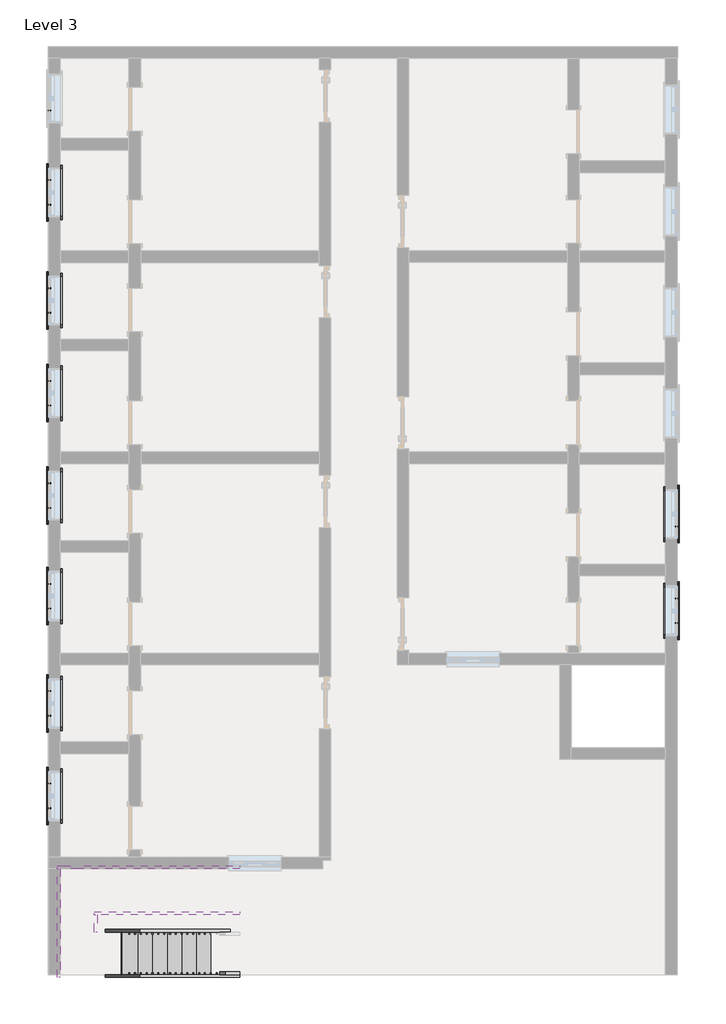
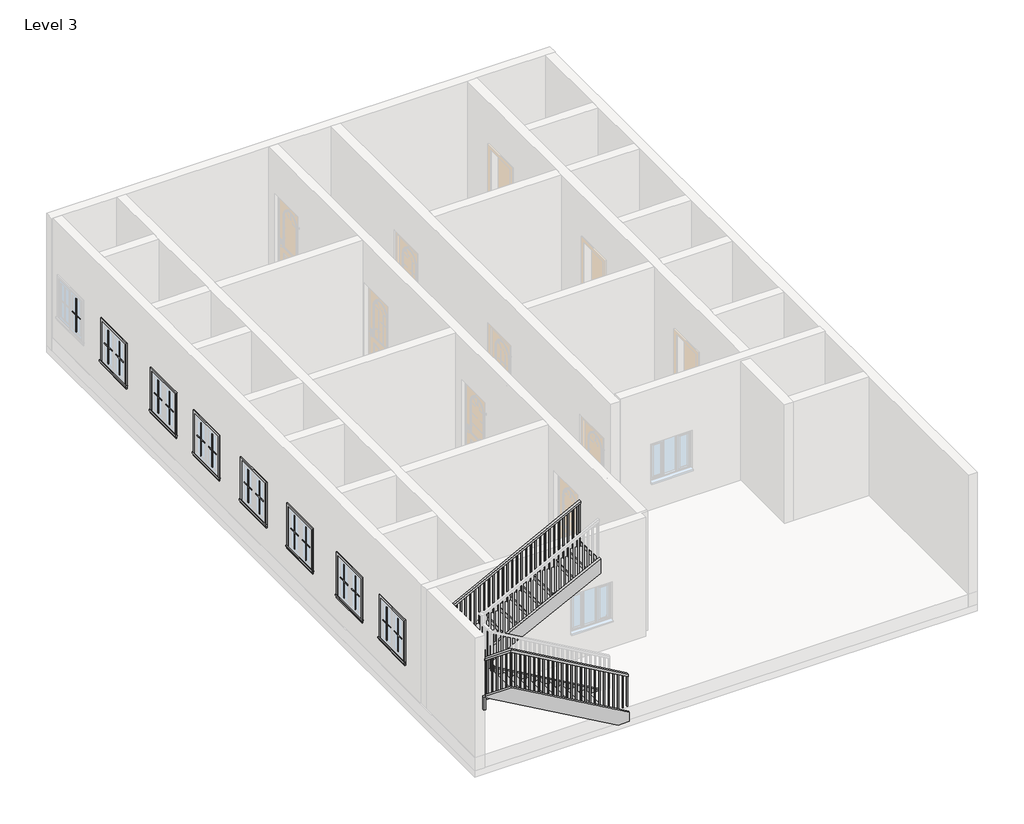
# One storey, part 3 of 4: 36 proxies, 6 members, 1 railing, 1 stair flight.
"""IFC4 building model written with IfcOpenShell, lengths in millimetres."""

from ifc_helpers import new_model, si_unit, frame, origin, place, context, project, spatial, polyline, outline, extrude, faceted_brep, transform, mapped, element, save
from components import muntin_pattern_2x2_muntin_pattern_2x2_b3fe6957, muntin_pattern_2x2_muntin_pattern_2x2_3e0ecaf2, trim_window_exterior_flat_with_sill_41619996, trim_window_interior_flat_picture_frame_51c85655, stair_flight_d547b7c1

model = new_model("IFC4")

# Units and contexts
model_context = context("Model", 3, world=origin())
ifc_project = project(units=[si_unit("LENGTHUNIT", "METRE", prefix="MILLI")], contexts=[model_context])

# Site, building, storey
site = spatial("IfcSite", under=ifc_project)
building = spatial("IfcBuilding", under=site)
storey = spatial("IfcBuildingStorey", under=building, Name="Level 3", Elevation=6096.0)

# Proxies
placement = place(None, origin())
muntin_pattern_2x2_muntin_pattern_2x2_shape = muntin_pattern_2x2_muntin_pattern_2x2_b3fe6957(model_context)
element("IfcBuildingElementProxy", 1, Name="Muntin Pattern_2x2 : Muntin Pattern_2x2", ObjectType="Muntin Pattern_2x2 : Muntin Pattern_2x2", at=placement, inside=storey, context=model_context, shape_type="MappedRepresentation", body=[
    mapped(muntin_pattern_2x2_muntin_pattern_2x2_shape, transform((-6438.8858866, 6882.8274728, 7080.25), x_axis=(0.0, 1.0, 0.0), y_axis=(-1.0, 0.0, 0.0), z_axis=(0.0, 0.0, 1.0))),
])
element("IfcBuildingElementProxy", 2, Name="Muntin Pattern_2x2 : Muntin Pattern_2x2", ObjectType="Muntin Pattern_2x2 : Muntin Pattern_2x2", at=placement, inside=storey, context=model_context, shape_type="MappedRepresentation", body=[
    mapped(muntin_pattern_2x2_muntin_pattern_2x2_shape, transform((-6438.8858866, 5244.5274728, 7080.25), x_axis=(0.0, 1.0, 0.0), y_axis=(-1.0, 0.0, 0.0), z_axis=(0.0, 0.0, 1.0))),
])
element("IfcBuildingElementProxy", 3, Name="Muntin Pattern_2x2 : Muntin Pattern_2x2", ObjectType="Muntin Pattern_2x2 : Muntin Pattern_2x2", at=placement, inside=storey, context=model_context, shape_type="MappedRepresentation", body=[
    mapped(muntin_pattern_2x2_muntin_pattern_2x2_shape, transform((-6438.8858866, 3360.4810874, 7080.25), x_axis=(0.0, 1.0, 0.0), y_axis=(-1.0, 0.0, 0.0), z_axis=(0.0, 0.0, 1.0))),
])
element("IfcBuildingElementProxy", 4, Name="Muntin Pattern_2x2 : Muntin Pattern_2x2", ObjectType="Muntin Pattern_2x2 : Muntin Pattern_2x2", at=placement, inside=storey, context=model_context, shape_type="MappedRepresentation", body=[
    mapped(muntin_pattern_2x2_muntin_pattern_2x2_shape, transform((-6438.8858866, 1745.426343, 7080.25), x_axis=(0.0, 1.0, 0.0), y_axis=(-1.0, 0.0, 0.0), z_axis=(0.0, 0.0, 1.0))),
])
element("IfcBuildingElementProxy", 5, Name="Muntin Pattern_2x2 : Muntin Pattern_2x2", ObjectType="Muntin Pattern_2x2 : Muntin Pattern_2x2", at=placement, inside=storey, context=model_context, shape_type="MappedRepresentation", body=[
    mapped(muntin_pattern_2x2_muntin_pattern_2x2_shape, transform((-6438.8858866, -38.6725272, 7080.25), x_axis=(0.0, 1.0, 0.0), y_axis=(-1.0, 0.0, 0.0), z_axis=(0.0, 0.0, 1.0))),
])
element("IfcBuildingElementProxy", 6, Name="Muntin Pattern_2x2 : Muntin Pattern_2x2", ObjectType="Muntin Pattern_2x2 : Muntin Pattern_2x2", at=placement, inside=storey, context=model_context, shape_type="MappedRepresentation", body=[
    mapped(muntin_pattern_2x2_muntin_pattern_2x2_shape, transform((-6438.8858866, -1791.2725272, 7080.25), x_axis=(0.0, 1.0, 0.0), y_axis=(-1.0, 0.0, 0.0), z_axis=(0.0, 0.0, 1.0))),
])
element("IfcBuildingElementProxy", 7, Name="Muntin Pattern_2x2 : Muntin Pattern_2x2", ObjectType="Muntin Pattern_2x2 : Muntin Pattern_2x2", at=placement, inside=storey, context=model_context, shape_type="MappedRepresentation", body=[
    mapped(muntin_pattern_2x2_muntin_pattern_2x2_shape, transform((-6438.8858866, -3658.1725272, 7080.25), x_axis=(0.0, 1.0, 0.0), y_axis=(-1.0, 0.0, 0.0), z_axis=(0.0, 0.0, 1.0))),
])
element("IfcBuildingElementProxy", 8, Name="Muntin Pattern_2x2 : Muntin Pattern_2x2", ObjectType="Muntin Pattern_2x2 : Muntin Pattern_2x2", at=placement, inside=storey, context=model_context, shape_type="MappedRepresentation", body=[
    mapped(muntin_pattern_2x2_muntin_pattern_2x2_shape, transform((-6438.8858866, -5271.0725272, 7080.25), x_axis=(0.0, 1.0, 0.0), y_axis=(-1.0, 0.0, 0.0), z_axis=(0.0, 0.0, 1.0))),
])
element("IfcBuildingElementProxy", 9, Name="Muntin Pattern_2x2 : Muntin Pattern_2x2", ObjectType="Muntin Pattern_2x2 : Muntin Pattern_2x2", at=placement, inside=storey, context=model_context, shape_type="MappedRepresentation", body=[
    mapped(muntin_pattern_2x2_muntin_pattern_2x2_shape, transform((4489.4641134, -1616.6475272, 7080.25), x_axis=(0.0, -1.0, 0.0), y_axis=(1.0, 0.0, 0.0), z_axis=(0.0, 0.0, 1.0))),
])
muntin_pattern_2x2_muntin_pattern_2x2_2_shape = muntin_pattern_2x2_muntin_pattern_2x2_3e0ecaf2(model_context)
element("IfcBuildingElementProxy", 10, Name="Muntin Pattern_2x2 : Muntin Pattern_2x2", ObjectType="Muntin Pattern_2x2 : Muntin Pattern_2x2", at=placement, inside=storey, context=model_context, shape_type="MappedRepresentation", body=[
    mapped(muntin_pattern_2x2_muntin_pattern_2x2_2_shape, transform((-6438.8858866, 5673.1524728, 7080.25), x_axis=(0.0, -1.0, 0.0), y_axis=(1.0, 0.0, 0.0), z_axis=(0.0, 0.0, 1.0))),
])
element("IfcBuildingElementProxy", 11, Name="Muntin Pattern_2x2 : Muntin Pattern_2x2", ObjectType="Muntin Pattern_2x2 : Muntin Pattern_2x2", at=placement, inside=storey, context=model_context, shape_type="MappedRepresentation", body=[
    mapped(muntin_pattern_2x2_muntin_pattern_2x2_2_shape, transform((-6438.8858866, 3789.1060874, 7080.25), x_axis=(0.0, -1.0, 0.0), y_axis=(1.0, 0.0, 0.0), z_axis=(0.0, 0.0, 1.0))),
])
element("IfcBuildingElementProxy", 12, Name="Muntin Pattern_2x2 : Muntin Pattern_2x2", ObjectType="Muntin Pattern_2x2 : Muntin Pattern_2x2", at=placement, inside=storey, context=model_context, shape_type="MappedRepresentation", body=[
    mapped(muntin_pattern_2x2_muntin_pattern_2x2_2_shape, transform((-6438.8858866, 2174.051343, 7080.25), x_axis=(0.0, -1.0, 0.0), y_axis=(1.0, 0.0, 0.0), z_axis=(0.0, 0.0, 1.0))),
])
element("IfcBuildingElementProxy", 13, Name="Muntin Pattern_2x2 : Muntin Pattern_2x2", ObjectType="Muntin Pattern_2x2 : Muntin Pattern_2x2", at=placement, inside=storey, context=model_context, shape_type="MappedRepresentation", body=[
    mapped(muntin_pattern_2x2_muntin_pattern_2x2_2_shape, transform((-6438.8858866, 389.9524728, 7080.25), x_axis=(0.0, -1.0, 0.0), y_axis=(1.0, 0.0, 0.0), z_axis=(0.0, 0.0, 1.0))),
])
element("IfcBuildingElementProxy", 14, Name="Muntin Pattern_2x2 : Muntin Pattern_2x2", ObjectType="Muntin Pattern_2x2 : Muntin Pattern_2x2", at=placement, inside=storey, context=model_context, shape_type="MappedRepresentation", body=[
    mapped(muntin_pattern_2x2_muntin_pattern_2x2_2_shape, transform((-6438.8858866, -1362.6475272, 7080.25), x_axis=(0.0, -1.0, 0.0), y_axis=(1.0, 0.0, 0.0), z_axis=(0.0, 0.0, 1.0))),
])
element("IfcBuildingElementProxy", 15, Name="Muntin Pattern_2x2 : Muntin Pattern_2x2", ObjectType="Muntin Pattern_2x2 : Muntin Pattern_2x2", at=placement, inside=storey, context=model_context, shape_type="MappedRepresentation", body=[
    mapped(muntin_pattern_2x2_muntin_pattern_2x2_2_shape, transform((-6438.8858866, -3229.5475272, 7080.25), x_axis=(0.0, -1.0, 0.0), y_axis=(1.0, 0.0, 0.0), z_axis=(0.0, 0.0, 1.0))),
])
element("IfcBuildingElementProxy", 16, Name="Muntin Pattern_2x2 : Muntin Pattern_2x2", ObjectType="Muntin Pattern_2x2 : Muntin Pattern_2x2", at=placement, inside=storey, context=model_context, shape_type="MappedRepresentation", body=[
    mapped(muntin_pattern_2x2_muntin_pattern_2x2_2_shape, transform((-6438.8858866, -4842.4475272, 7080.25), x_axis=(0.0, -1.0, 0.0), y_axis=(1.0, 0.0, 0.0), z_axis=(0.0, 0.0, 1.0))),
])
element("IfcBuildingElementProxy", 17, Name="Muntin Pattern_2x2 : Muntin Pattern_2x2", ObjectType="Muntin Pattern_2x2 : Muntin Pattern_2x2", at=placement, inside=storey, context=model_context, shape_type="MappedRepresentation", body=[
    mapped(muntin_pattern_2x2_muntin_pattern_2x2_2_shape, transform((4489.4641134, -2045.2725272, 7080.25), x_axis=(0.0, 1.0, 0.0), y_axis=(-1.0, 0.0, 0.0), z_axis=(0.0, 0.0, 1.0))),
])
element("IfcBuildingElementProxy", 18, Name="Muntin Pattern_2x2 : Muntin Pattern_2x2", ObjectType="Muntin Pattern_2x2 : Muntin Pattern_2x2", at=placement, inside=storey, context=model_context, shape_type="MappedRepresentation", body=[
    mapped(muntin_pattern_2x2_muntin_pattern_2x2_2_shape, transform((4489.4641134, -362.5225272, 7080.25), x_axis=(0.0, 1.0, 0.0), y_axis=(-1.0, 0.0, 0.0), z_axis=(0.0, 0.0, 1.0))),
])
trim_window_exterior_flat_with_sill_shape = trim_window_exterior_flat_with_sill_41619996(model_context)
element("IfcBuildingElementProxy", 19, Name="Trim-Window-Exterior-Flat : with Sill", ObjectType="Trim-Window-Exterior-Flat : with Sill", at=placement, inside=storey, context=model_context, shape_type="MappedRepresentation", body=[
    mapped(trim_window_exterior_flat_with_sill_shape, transform((-6448.4108866, 5458.8399728, 7924.8), x_axis=(0.0, -1.0, 0.0), y_axis=(0.0, 0.0, 1.0), z_axis=(-1.0, 0.0, 0.0))),
])
element("IfcBuildingElementProxy", 20, Name="Trim-Window-Exterior-Flat : with Sill", ObjectType="Trim-Window-Exterior-Flat : with Sill", at=placement, inside=storey, context=model_context, shape_type="MappedRepresentation", body=[
    mapped(trim_window_exterior_flat_with_sill_shape, transform((-6448.4108866, 3574.7935874, 7924.8), x_axis=(0.0, -1.0, 0.0), y_axis=(0.0, 0.0, 1.0), z_axis=(-1.0, 0.0, 0.0))),
])
element("IfcBuildingElementProxy", 21, Name="Trim-Window-Exterior-Flat : with Sill", ObjectType="Trim-Window-Exterior-Flat : with Sill", at=placement, inside=storey, context=model_context, shape_type="MappedRepresentation", body=[
    mapped(trim_window_exterior_flat_with_sill_shape, transform((-6448.4108866, 1959.738843, 7924.8), x_axis=(0.0, -1.0, 0.0), y_axis=(0.0, 0.0, 1.0), z_axis=(-1.0, 0.0, 0.0))),
])
element("IfcBuildingElementProxy", 22, Name="Trim-Window-Exterior-Flat : with Sill", ObjectType="Trim-Window-Exterior-Flat : with Sill", at=placement, inside=storey, context=model_context, shape_type="MappedRepresentation", body=[
    mapped(trim_window_exterior_flat_with_sill_shape, transform((-6448.4108866, 175.6399728, 7924.8), x_axis=(0.0, -1.0, 0.0), y_axis=(0.0, 0.0, 1.0), z_axis=(-1.0, 0.0, 0.0))),
])
element("IfcBuildingElementProxy", 23, Name="Trim-Window-Exterior-Flat : with Sill", ObjectType="Trim-Window-Exterior-Flat : with Sill", at=placement, inside=storey, context=model_context, shape_type="MappedRepresentation", body=[
    mapped(trim_window_exterior_flat_with_sill_shape, transform((-6448.4108866, -1576.9600272, 7924.8), x_axis=(0.0, -1.0, 0.0), y_axis=(0.0, 0.0, 1.0), z_axis=(-1.0, 0.0, 0.0))),
])
element("IfcBuildingElementProxy", 24, Name="Trim-Window-Exterior-Flat : with Sill", ObjectType="Trim-Window-Exterior-Flat : with Sill", at=placement, inside=storey, context=model_context, shape_type="MappedRepresentation", body=[
    mapped(trim_window_exterior_flat_with_sill_shape, transform((-6448.4108866, -3443.8600272, 7924.8), x_axis=(0.0, -1.0, 0.0), y_axis=(0.0, 0.0, 1.0), z_axis=(-1.0, 0.0, 0.0))),
])
element("IfcBuildingElementProxy", 25, Name="Trim-Window-Exterior-Flat : with Sill", ObjectType="Trim-Window-Exterior-Flat : with Sill", at=placement, inside=storey, context=model_context, shape_type="MappedRepresentation", body=[
    mapped(trim_window_exterior_flat_with_sill_shape, transform((-6448.4108866, -5056.7600272, 7924.8), x_axis=(0.0, -1.0, 0.0), y_axis=(0.0, 0.0, 1.0), z_axis=(-1.0, 0.0, 0.0))),
])
element("IfcBuildingElementProxy", 26, Name="Trim-Window-Exterior-Flat : with Sill", ObjectType="Trim-Window-Exterior-Flat : with Sill", at=placement, inside=storey, context=model_context, shape_type="MappedRepresentation", body=[
    mapped(trim_window_exterior_flat_with_sill_shape, transform((4498.9891134, -1830.9600272, 7924.8), x_axis=(0.0, 1.0, 0.0), y_axis=(0.0, 0.0, 1.0), z_axis=(1.0, 0.0, 0.0))),
])
element("IfcBuildingElementProxy", 27, Name="Trim-Window-Exterior-Flat : with Sill", ObjectType="Trim-Window-Exterior-Flat : with Sill", at=placement, inside=storey, context=model_context, shape_type="MappedRepresentation", body=[
    mapped(trim_window_exterior_flat_with_sill_shape, transform((4498.9891134, -148.2100272, 7924.8), x_axis=(0.0, 1.0, 0.0), y_axis=(0.0, 0.0, 1.0), z_axis=(1.0, 0.0, 0.0))),
])
trim_window_interior_flat_picture_frame_shape = trim_window_interior_flat_picture_frame_51c85655(model_context)
element("IfcBuildingElementProxy", 28, Name="Trim-Window-Interior-Flat : Picture Frame", ObjectType="Trim-Window-Interior-Flat : Picture Frame", at=placement, inside=storey, context=model_context, shape_type="MappedRepresentation", body=[
    mapped(trim_window_interior_flat_picture_frame_shape, transform((-6245.2108866, 5458.8399728, 7924.8), x_axis=(0.0, 1.0, 0.0), y_axis=(0.0, 0.0, 1.0), z_axis=(1.0, 0.0, 0.0))),
])
element("IfcBuildingElementProxy", 29, Name="Trim-Window-Interior-Flat : Picture Frame", ObjectType="Trim-Window-Interior-Flat : Picture Frame", at=placement, inside=storey, context=model_context, shape_type="MappedRepresentation", body=[
    mapped(trim_window_interior_flat_picture_frame_shape, transform((-6245.2108866, 3574.7935874, 7924.8), x_axis=(0.0, 1.0, 0.0), y_axis=(0.0, 0.0, 1.0), z_axis=(1.0, 0.0, 0.0))),
])
element("IfcBuildingElementProxy", 30, Name="Trim-Window-Interior-Flat : Picture Frame", ObjectType="Trim-Window-Interior-Flat : Picture Frame", at=placement, inside=storey, context=model_context, shape_type="MappedRepresentation", body=[
    mapped(trim_window_interior_flat_picture_frame_shape, transform((-6245.2108866, 1959.738843, 7924.8), x_axis=(0.0, 1.0, 0.0), y_axis=(0.0, 0.0, 1.0), z_axis=(1.0, 0.0, 0.0))),
])
element("IfcBuildingElementProxy", 31, Name="Trim-Window-Interior-Flat : Picture Frame", ObjectType="Trim-Window-Interior-Flat : Picture Frame", at=placement, inside=storey, context=model_context, shape_type="MappedRepresentation", body=[
    mapped(trim_window_interior_flat_picture_frame_shape, transform((-6245.2108866, 175.6399728, 7924.8), x_axis=(0.0, 1.0, 0.0), y_axis=(0.0, 0.0, 1.0), z_axis=(1.0, 0.0, 0.0))),
])
element("IfcBuildingElementProxy", 32, Name="Trim-Window-Interior-Flat : Picture Frame", ObjectType="Trim-Window-Interior-Flat : Picture Frame", at=placement, inside=storey, context=model_context, shape_type="MappedRepresentation", body=[
    mapped(trim_window_interior_flat_picture_frame_shape, transform((-6245.2108866, -1576.9600272, 7924.8), x_axis=(0.0, 1.0, 0.0), y_axis=(0.0, 0.0, 1.0), z_axis=(1.0, 0.0, 0.0))),
])
element("IfcBuildingElementProxy", 33, Name="Trim-Window-Interior-Flat : Picture Frame", ObjectType="Trim-Window-Interior-Flat : Picture Frame", at=placement, inside=storey, context=model_context, shape_type="MappedRepresentation", body=[
    mapped(trim_window_interior_flat_picture_frame_shape, transform((-6245.2108866, -3443.8600272, 7924.8), x_axis=(0.0, 1.0, 0.0), y_axis=(0.0, 0.0, 1.0), z_axis=(1.0, 0.0, 0.0))),
])
element("IfcBuildingElementProxy", 34, Name="Trim-Window-Interior-Flat : Picture Frame", ObjectType="Trim-Window-Interior-Flat : Picture Frame", at=placement, inside=storey, context=model_context, shape_type="MappedRepresentation", body=[
    mapped(trim_window_interior_flat_picture_frame_shape, transform((-6245.2108866, -5056.7600272, 7924.8), x_axis=(0.0, 1.0, 0.0), y_axis=(0.0, 0.0, 1.0), z_axis=(1.0, 0.0, 0.0))),
])
element("IfcBuildingElementProxy", 35, Name="Trim-Window-Interior-Flat : Picture Frame", ObjectType="Trim-Window-Interior-Flat : Picture Frame", at=placement, inside=storey, context=model_context, shape_type="MappedRepresentation", body=[
    mapped(trim_window_interior_flat_picture_frame_shape, transform((4295.7891134, -1830.9600272, 7924.8), x_axis=(0.0, -1.0, 0.0), y_axis=(0.0, 0.0, 1.0), z_axis=(-1.0, 0.0, 0.0))),
])
element("IfcBuildingElementProxy", 36, Name="Trim-Window-Interior-Flat : Picture Frame", ObjectType="Trim-Window-Interior-Flat : Picture Frame", at=placement, inside=storey, context=model_context, shape_type="MappedRepresentation", body=[
    mapped(trim_window_interior_flat_picture_frame_shape, transform((4295.7891134, -148.2100272, 7924.8), x_axis=(0.0, -1.0, 0.0), y_axis=(0.0, 0.0, 1.0), z_axis=(-1.0, 0.0, 0.0))),
])

# Members
element("IfcMember", 37, ObjectType="Stringer - 2\" Width", at=placement, inside=storey, context=model_context, shape_type="SweptSolid", body=[
    extrude(outline(polyline([(6096.0, -3117.2664982), (6304.974685, -3117.2664982), (7768.7714286, -5678.9107995), (7768.7714286, -6245.2108866), (7741.3177409, -6245.2108866), (6096.0, -3365.9048399), (6096.0, -3117.2664982)])), frame((0.0, -8219.0600272, 0.0), z_axis=(0.0, 1.0, 0.0), x_axis=(0.0, 0.0, 1.0)), (0.0, 0.0, 1.0), 50.8),
])
element("IfcMember", 38, ObjectType="Stringer - 2\" Width", at=placement, inside=storey, context=model_context, shape_type="SweptSolid", body=[
    extrude(outline(polyline([(-6245.2108866, -8219.0600272), (-6296.0108866, -8219.0600272), (-6296.0108866, -6326.7600272), (-6245.2108866, -6326.7600272), (-6245.2108866, -8219.0600272)])), frame((0.0, 0.0, 7463.9714286), z_axis=(0.0, 0.0, 1.0), x_axis=(1.0, 0.0, 0.0)), (0.0, 0.0, 1.0), 304.8),
])
element("IfcMember", 39, ObjectType="Stringer - 2\" Width", at=placement, inside=storey, context=model_context, shape_type="SweptSolid", body=[
    extrude(outline(polyline([(7571.8463219, -6296.0108866), (7463.9714286, -6296.0108866), (7463.9714286, -5835.3420022), (8844.5812084, -3117.2664982), (9186.4466461, -3117.2664982), (7571.8463219, -6296.0108866)])), frame((0.0, -6326.7600272, 0.0), z_axis=(0.0, 1.0, 0.0), x_axis=(0.0, 0.0, 1.0)), (0.0, 0.0, 1.0), 50.8),
])
element("IfcMember", 40, ObjectType="Stringer - 2\" Width", at=placement, inside=storey, context=model_context, shape_type="SweptSolid", body=[
    extrude(outline(polyline([(6096.0, -3117.2664982), (6304.974685, -3117.2664982), (7727.374685, -5606.4664982), (7376.3209476, -5606.4664982), (6096.0, -3365.9048399), (6096.0, -3117.2664982)])), frame((0.0, -7431.6600272, 0.0), z_axis=(0.0, 1.0, 0.0), x_axis=(0.0, 0.0, 1.0)), (0.0, 0.0, 1.0), 50.8),
])
element("IfcMember", 41, ObjectType="Stringer - 2\" Width", at=placement, inside=storey, context=model_context, shape_type="SweptSolid", body=[
    extrude(outline(polyline([(-5606.4664982, -7431.6600272), (-5657.2664982, -7431.6600272), (-5657.2664982, -7126.8600272), (-5606.4664982, -7126.8600272), (-5606.4664982, -7431.6600272)])), frame((0.0, 0.0, 7463.9714286), z_axis=(0.0, 0.0, 1.0), x_axis=(1.0, 0.0, 0.0)), (0.0, 0.0, 1.0), 304.8),
])
element("IfcMember", 42, ObjectType="Stringer - 2\" Width", at=placement, inside=storey, context=model_context, shape_type="SweptSolid", body=[
    extrude(outline(polyline([(7896.287916, -5657.2664982), (7554.4224783, -5657.2664982), (8844.5812084, -3117.2664982), (9186.4466461, -3117.2664982), (7896.287916, -5657.2664982)])), frame((0.0, -7126.8600272, 0.0), z_axis=(0.0, 1.0, 0.0), x_axis=(0.0, 0.0, 1.0)), (0.0, 0.0, 1.0), 50.8),
])

# Railing
element("IfcRailing", 43, ObjectType="Handrail - Rectangular", at=placement, inside=storey, context=model_context, shape_type="SolidModel", body=[
    faceted_brep([(-3117.2664982, -8168.2600272, 7155.5428571), (-3117.2664982, -8168.2600272, 7097.0339009), (-3117.2664982, -8117.4600272, 7097.0339009), (-3117.2664982, -8117.4600272, 7155.5428571), (-5657.2664982, -8168.2600272, 8606.9714286), (-5670.7571716, -8168.2600272, 8556.1714286), (-5670.7571716, -8117.4600272, 8556.1714286), (-5657.2664982, -8117.4600272, 8606.9714286), (-6245.2108866, -8168.2600272, 8606.9714286), (-6245.2108866, -8168.2600272, 8556.1714286), (-6194.4108866, -8117.4600272, 8556.1714286), (-6194.4108866, -8117.4600272, 8606.9714286), (-6245.2108866, -6326.7600272, 8606.9714286), (-6245.2108866, -6326.7600272, 8556.1714286), (-6194.4108866, -6377.5600272, 8556.1714286), (-6194.4108866, -6377.5600272, 8606.9714286), (-5939.4887204, -6326.7600272, 8606.9714286), (-5927.1913462, -6326.7600272, 8556.1714286), (-5927.1913462, -6377.5600272, 8556.1714286), (-5939.4887204, -6377.5600272, 8606.9714286), (-3117.2664982, -6326.7600272, 10058.4), (-3117.2664982, -6377.5600272, 10058.4), (-3117.2664982, -6377.5600272, 10001.2756361), (-3117.2664982, -6326.7600272, 10001.2756361)], [[[0, 1, 2, 3]], [[1, 0, 4, 5]], [[2, 1, 5, 6]], [[3, 2, 6, 7]], [[0, 3, 7, 4]], [[5, 4, 8, 9]], [[6, 5, 9, 10]], [[7, 6, 10, 11]], [[4, 7, 11, 8]], [[9, 8, 12, 13]], [[10, 9, 13, 14]], [[11, 10, 14, 15]], [[8, 11, 15, 12]], [[13, 12, 16, 17]], [[14, 13, 17, 18]], [[15, 14, 18, 19]], [[12, 15, 19, 16]], [[20, 21, 22, 23]], [[17, 16, 20, 23]], [[18, 17, 23, 22]], [[19, 18, 22, 21]], [[16, 19, 21, 20]]]),
    extrude(outline(polyline([(9968.325665, -3181.3358866), (8998.8571429, -3181.3358866), (8998.8571429, -3162.2858866), (9978.1228078, -3162.2858866), (9968.325665, -3181.3358866)])), frame((0.0, -6361.6850272, 0.0), z_axis=(0.0, 1.0, 0.0), x_axis=(0.0, 0.0, 1.0)), (0.0, 0.0, 1.0), 19.05),
    extrude(outline(polyline([(9916.0742364, -3282.9358866), (8998.8571429, -3282.9358866), (8998.8571429, -3263.8858866), (9925.8713793, -3263.8858866), (9916.0742364, -3282.9358866)])), frame((0.0, -6361.6850272, 0.0), z_axis=(0.0, 1.0, 0.0), x_axis=(0.0, 0.0, 1.0)), (0.0, 0.0, 1.0), 19.05),
    extrude(outline(polyline([(9863.8228078, -3384.5358866), (8853.7142857, -3384.5358866), (8853.7142857, -3365.4858866), (9873.6199507, -3365.4858866), (9863.8228078, -3384.5358866)])), frame((0.0, -6361.6850272, 0.0), z_axis=(0.0, 1.0, 0.0), x_axis=(0.0, 0.0, 1.0)), (0.0, 0.0, 1.0), 19.05),
    extrude(outline(polyline([(9811.5713793, -3486.1358866), (8853.7142857, -3486.1358866), (8853.7142857, -3467.0858866), (9821.3685221, -3467.0858866), (9811.5713793, -3486.1358866)])), frame((0.0, -6361.6850272, 0.0), z_axis=(0.0, 1.0, 0.0), x_axis=(0.0, 0.0, 1.0)), (0.0, 0.0, 1.0), 19.05),
    extrude(outline(polyline([(9759.3199507, -3587.7358866), (8853.7142857, -3587.7358866), (8853.7142857, -3568.6858866), (9769.1170935, -3568.6858866), (9759.3199507, -3587.7358866)])), frame((0.0, -6361.6850272, 0.0), z_axis=(0.0, 1.0, 0.0), x_axis=(0.0, 0.0, 1.0)), (0.0, 0.0, 1.0), 19.05),
    extrude(outline(polyline([(9707.0685221, -3689.3358866), (8708.5714286, -3689.3358866), (8708.5714286, -3670.2858866), (9716.865665, -3670.2858866), (9707.0685221, -3689.3358866)])), frame((0.0, -6361.6850272, 0.0), z_axis=(0.0, 1.0, 0.0), x_axis=(0.0, 0.0, 1.0)), (0.0, 0.0, 1.0), 19.05),
    extrude(outline(polyline([(9654.8170935, -3790.9358866), (8708.5714286, -3790.9358866), (8708.5714286, -3771.8858866), (9664.6142364, -3771.8858866), (9654.8170935, -3790.9358866)])), frame((0.0, -6361.6850272, 0.0), z_axis=(0.0, 1.0, 0.0), x_axis=(0.0, 0.0, 1.0)), (0.0, 0.0, 1.0), 19.05),
    extrude(outline(polyline([(9602.565665, -3892.5358866), (8708.5714286, -3892.5358866), (8708.5714286, -3873.4858866), (9612.3628078, -3873.4858866), (9602.565665, -3892.5358866)])), frame((0.0, -6361.6850272, 0.0), z_axis=(0.0, 1.0, 0.0), x_axis=(0.0, 0.0, 1.0)), (0.0, 0.0, 1.0), 19.05),
    extrude(outline(polyline([(9550.3142364, -3994.1358866), (8708.5714286, -3994.1358866), (8708.5714286, -3975.0858866), (9560.1113793, -3975.0858866), (9550.3142364, -3994.1358866)])), frame((0.0, -6361.6850272, 0.0), z_axis=(0.0, 1.0, 0.0), x_axis=(0.0, 0.0, 1.0)), (0.0, 0.0, 1.0), 19.05),
    extrude(outline(polyline([(9498.0628078, -4095.7358866), (8708.5714286, -4095.7358866), (8708.5714286, -4076.6858866), (9507.8599507, -4076.6858866), (9498.0628078, -4095.7358866)])), frame((0.0, -6361.6850272, 0.0), z_axis=(0.0, 1.0, 0.0), x_axis=(0.0, 0.0, 1.0)), (0.0, 0.0, 1.0), 19.05),
    extrude(outline(polyline([(9445.8113793, -4197.3358866), (8563.4285714, -4197.3358866), (8563.4285714, -4178.2858866), (9455.6085221, -4178.2858866), (9445.8113793, -4197.3358866)])), frame((0.0, -6361.6850272, 0.0), z_axis=(0.0, 1.0, 0.0), x_axis=(0.0, 0.0, 1.0)), (0.0, 0.0, 1.0), 19.05),
    extrude(outline(polyline([(9393.5599507, -4298.9358866), (8563.4285714, -4298.9358866), (8563.4285714, -4279.8858866), (9403.3570935, -4279.8858866), (9393.5599507, -4298.9358866)])), frame((0.0, -6361.6850272, 0.0), z_axis=(0.0, 1.0, 0.0), x_axis=(0.0, 0.0, 1.0)), (0.0, 0.0, 1.0), 19.05),
    extrude(outline(polyline([(9341.3085221, -4400.5358866), (8418.2857143, -4400.5358866), (8418.2857143, -4381.4858866), (9351.105665, -4381.4858866), (9341.3085221, -4400.5358866)])), frame((0.0, -6361.6850272, 0.0), z_axis=(0.0, 1.0, 0.0), x_axis=(0.0, 0.0, 1.0)), (0.0, 0.0, 1.0), 19.05),
    extrude(outline(polyline([(9289.0570935, -4502.1358866), (8418.2857143, -4502.1358866), (8418.2857143, -4483.0858866), (9298.8542364, -4483.0858866), (9289.0570935, -4502.1358866)])), frame((0.0, -6361.6850272, 0.0), z_axis=(0.0, 1.0, 0.0), x_axis=(0.0, 0.0, 1.0)), (0.0, 0.0, 1.0), 19.05),
    extrude(outline(polyline([(9236.805665, -4603.7358866), (8418.2857143, -4603.7358866), (8418.2857143, -4584.6858866), (9246.6028078, -4584.6858866), (9236.805665, -4603.7358866)])), frame((0.0, -6361.6850272, 0.0), z_axis=(0.0, 1.0, 0.0), x_axis=(0.0, 0.0, 1.0)), (0.0, 0.0, 1.0), 19.05),
    extrude(outline(polyline([(9184.5542364, -4705.3358866), (8273.1428571, -4705.3358866), (8273.1428571, -4686.2858866), (9194.3513793, -4686.2858866), (9184.5542364, -4705.3358866)])), frame((0.0, -6361.6850272, 0.0), z_axis=(0.0, 1.0, 0.0), x_axis=(0.0, 0.0, 1.0)), (0.0, 0.0, 1.0), 19.05),
    extrude(outline(polyline([(9132.3028078, -4806.9358866), (8273.1428571, -4806.9358866), (8273.1428571, -4787.8858866), (9142.0999507, -4787.8858866), (9132.3028078, -4806.9358866)])), frame((0.0, -6361.6850272, 0.0), z_axis=(0.0, 1.0, 0.0), x_axis=(0.0, 0.0, 1.0)), (0.0, 0.0, 1.0), 19.05),
    extrude(outline(polyline([(9080.0513793, -4908.5358866), (8128.0, -4908.5358866), (8128.0, -4889.4858866), (9089.8485221, -4889.4858866), (9080.0513793, -4908.5358866)])), frame((0.0, -6361.6850272, 0.0), z_axis=(0.0, 1.0, 0.0), x_axis=(0.0, 0.0, 1.0)), (0.0, 0.0, 1.0), 19.05),
    extrude(outline(polyline([(9027.7999507, -5010.1358866), (8128.0, -5010.1358866), (8128.0, -4991.0858866), (9037.5970935, -4991.0858866), (9027.7999507, -5010.1358866)])), frame((0.0, -6361.6850272, 0.0), z_axis=(0.0, 1.0, 0.0), x_axis=(0.0, 0.0, 1.0)), (0.0, 0.0, 1.0), 19.05),
    extrude(outline(polyline([(8975.5485221, -5111.7358866), (8128.0, -5111.7358866), (8128.0, -5092.6858866), (8985.345665, -5092.6858866), (8975.5485221, -5111.7358866)])), frame((0.0, -6361.6850272, 0.0), z_axis=(0.0, 1.0, 0.0), x_axis=(0.0, 0.0, 1.0)), (0.0, 0.0, 1.0), 19.05),
    extrude(outline(polyline([(8923.2970935, -5213.3358866), (7982.8571429, -5213.3358866), (7982.8571429, -5194.2858866), (8933.0942364, -5194.2858866), (8923.2970935, -5213.3358866)])), frame((0.0, -6361.6850272, 0.0), z_axis=(0.0, 1.0, 0.0), x_axis=(0.0, 0.0, 1.0)), (0.0, 0.0, 1.0), 19.05),
    extrude(outline(polyline([(8871.045665, -5314.9358866), (7982.8571429, -5314.9358866), (7982.8571429, -5295.8858866), (8880.8428078, -5295.8858866), (8871.045665, -5314.9358866)])), frame((0.0, -6361.6850272, 0.0), z_axis=(0.0, 1.0, 0.0), x_axis=(0.0, 0.0, 1.0)), (0.0, 0.0, 1.0), 19.05),
    extrude(outline(polyline([(8818.7942364, -5416.5358866), (7837.7142857, -5416.5358866), (7837.7142857, -5397.4858866), (8828.5913793, -5397.4858866), (8818.7942364, -5416.5358866)])), frame((0.0, -6361.6850272, 0.0), z_axis=(0.0, 1.0, 0.0), x_axis=(0.0, 0.0, 1.0)), (0.0, 0.0, 1.0), 19.05),
    extrude(outline(polyline([(8766.5428078, -5518.1358866), (7837.7142857, -5518.1358866), (7837.7142857, -5499.0858866), (8776.3399507, -5499.0858866), (8766.5428078, -5518.1358866)])), frame((0.0, -6361.6850272, 0.0), z_axis=(0.0, 1.0, 0.0), x_axis=(0.0, 0.0, 1.0)), (0.0, 0.0, 1.0), 19.05),
    extrude(outline(polyline([(8714.2913793, -5619.7358866), (7837.7142857, -5619.7358866), (7837.7142857, -5600.6858866), (8724.0885221, -5600.6858866), (8714.2913793, -5619.7358866)])), frame((0.0, -6361.6850272, 0.0), z_axis=(0.0, 1.0, 0.0), x_axis=(0.0, 0.0, 1.0)), (0.0, 0.0, 1.0), 19.05),
    extrude(outline(polyline([(8662.0399507, -5721.3358866), (7692.5714286, -5721.3358866), (7692.5714286, -5702.2858866), (8671.8370935, -5702.2858866), (8662.0399507, -5721.3358866)])), frame((0.0, -6361.6850272, 0.0), z_axis=(0.0, 1.0, 0.0), x_axis=(0.0, 0.0, 1.0)), (0.0, 0.0, 1.0), 19.05),
    extrude(outline(polyline([(8609.7885221, -5822.9358866), (7692.5714286, -5822.9358866), (7692.5714286, -5803.8858866), (8619.585665, -5803.8858866), (8609.7885221, -5822.9358866)])), frame((0.0, -6361.6850272, 0.0), z_axis=(0.0, 1.0, 0.0), x_axis=(0.0, 0.0, 1.0)), (0.0, 0.0, 1.0), 19.05),
    extrude(outline(polyline([(8557.5370935, -5924.5358866), (7692.5714286, -5924.5358866), (7692.5714286, -5905.4858866), (8567.3342364, -5905.4858866), (8557.5370935, -5924.5358866)])), frame((0.0, -6361.6850272, 0.0), z_axis=(0.0, 1.0, 0.0), x_axis=(0.0, 0.0, 1.0)), (0.0, 0.0, 1.0), 19.05),
    extrude(outline(polyline([(-6026.1358866, -6342.6350272), (-6007.0858866, -6342.6350272), (-6007.0858866, -6361.6850272), (-6026.1358866, -6361.6850272), (-6026.1358866, -6342.6350272)])), frame((0.0, 0.0, 7692.5714286), z_axis=(0.0, 0.0, 1.0), x_axis=(1.0, 0.0, 0.0)), (0.0, 0.0, 1.0), 863.6),
    extrude(outline(polyline([(-6127.7358866, -6342.6350272), (-6108.6858866, -6342.6350272), (-6108.6858866, -6361.6850272), (-6127.7358866, -6361.6850272), (-6127.7358866, -6342.6350272)])), frame((0.0, 0.0, 7692.5714286), z_axis=(0.0, 0.0, 1.0), x_axis=(1.0, 0.0, 0.0)), (0.0, 0.0, 1.0), 863.6),
    extrude(outline(polyline([(-6229.3358866, -6425.1850272), (-6229.3358866, -6406.1350272), (-6210.2858866, -6406.1350272), (-6210.2858866, -6425.1850272), (-6229.3358866, -6425.1850272)])), frame((0.0, 0.0, 7692.5714286), z_axis=(0.0, 0.0, 1.0), x_axis=(1.0, 0.0, 0.0)), (0.0, 0.0, 1.0), 863.6),
    extrude(outline(polyline([(-6229.3358866, -6526.7850272), (-6229.3358866, -6507.7350272), (-6210.2858866, -6507.7350272), (-6210.2858866, -6526.7850272), (-6229.3358866, -6526.7850272)])), frame((0.0, 0.0, 7692.5714286), z_axis=(0.0, 0.0, 1.0), x_axis=(1.0, 0.0, 0.0)), (0.0, 0.0, 1.0), 863.6),
    extrude(outline(polyline([(-6229.3358866, -6628.3850272), (-6229.3358866, -6609.3350272), (-6210.2858866, -6609.3350272), (-6210.2858866, -6628.3850272), (-6229.3358866, -6628.3850272)])), frame((0.0, 0.0, 7692.5714286), z_axis=(0.0, 0.0, 1.0), x_axis=(1.0, 0.0, 0.0)), (0.0, 0.0, 1.0), 863.6),
    extrude(outline(polyline([(-6229.3358866, -6729.9850272), (-6229.3358866, -6710.9350272), (-6210.2858866, -6710.9350272), (-6210.2858866, -6729.9850272), (-6229.3358866, -6729.9850272)])), frame((0.0, 0.0, 7692.5714286), z_axis=(0.0, 0.0, 1.0), x_axis=(1.0, 0.0, 0.0)), (0.0, 0.0, 1.0), 863.6),
    extrude(outline(polyline([(-6229.3358866, -6831.5850272), (-6229.3358866, -6812.5350272), (-6210.2858866, -6812.5350272), (-6210.2858866, -6831.5850272), (-6229.3358866, -6831.5850272)])), frame((0.0, 0.0, 7692.5714286), z_axis=(0.0, 0.0, 1.0), x_axis=(1.0, 0.0, 0.0)), (0.0, 0.0, 1.0), 863.6),
    extrude(outline(polyline([(-6229.3358866, -6933.1850272), (-6229.3358866, -6914.1350272), (-6210.2858866, -6914.1350272), (-6210.2858866, -6933.1850272), (-6229.3358866, -6933.1850272)])), frame((0.0, 0.0, 7692.5714286), z_axis=(0.0, 0.0, 1.0), x_axis=(1.0, 0.0, 0.0)), (0.0, 0.0, 1.0), 863.6),
    extrude(outline(polyline([(-6229.3358866, -7034.7850272), (-6229.3358866, -7015.7350272), (-6210.2858866, -7015.7350272), (-6210.2858866, -7034.7850272), (-6229.3358866, -7034.7850272)])), frame((0.0, 0.0, 7692.5714286), z_axis=(0.0, 0.0, 1.0), x_axis=(1.0, 0.0, 0.0)), (0.0, 0.0, 1.0), 863.6),
    extrude(outline(polyline([(-6229.3358866, -7136.3850272), (-6229.3358866, -7117.3350272), (-6210.2858866, -7117.3350272), (-6210.2858866, -7136.3850272), (-6229.3358866, -7136.3850272)])), frame((0.0, 0.0, 7692.5714286), z_axis=(0.0, 0.0, 1.0), x_axis=(1.0, 0.0, 0.0)), (0.0, 0.0, 1.0), 863.6),
    extrude(outline(polyline([(-6229.3358866, -7237.9850272), (-6229.3358866, -7218.9350272), (-6210.2858866, -7218.9350272), (-6210.2858866, -7237.9850272), (-6229.3358866, -7237.9850272)])), frame((0.0, 0.0, 7692.5714286), z_axis=(0.0, 0.0, 1.0), x_axis=(1.0, 0.0, 0.0)), (0.0, 0.0, 1.0), 863.6),
    extrude(outline(polyline([(-6229.3358866, -7339.5850272), (-6229.3358866, -7320.5350272), (-6210.2858866, -7320.5350272), (-6210.2858866, -7339.5850272), (-6229.3358866, -7339.5850272)])), frame((0.0, 0.0, 7692.5714286), z_axis=(0.0, 0.0, 1.0), x_axis=(1.0, 0.0, 0.0)), (0.0, 0.0, 1.0), 863.6),
    extrude(outline(polyline([(-6229.3358866, -7441.1850272), (-6229.3358866, -7422.1350272), (-6210.2858866, -7422.1350272), (-6210.2858866, -7441.1850272), (-6229.3358866, -7441.1850272)])), frame((0.0, 0.0, 7692.5714286), z_axis=(0.0, 0.0, 1.0), x_axis=(1.0, 0.0, 0.0)), (0.0, 0.0, 1.0), 863.6),
    extrude(outline(polyline([(-6229.3358866, -7542.7850272), (-6229.3358866, -7523.7350272), (-6210.2858866, -7523.7350272), (-6210.2858866, -7542.7850272), (-6229.3358866, -7542.7850272)])), frame((0.0, 0.0, 7692.5714286), z_axis=(0.0, 0.0, 1.0), x_axis=(1.0, 0.0, 0.0)), (0.0, 0.0, 1.0), 863.6),
    extrude(outline(polyline([(-6229.3358866, -7644.3850272), (-6229.3358866, -7625.3350272), (-6210.2858866, -7625.3350272), (-6210.2858866, -7644.3850272), (-6229.3358866, -7644.3850272)])), frame((0.0, 0.0, 7692.5714286), z_axis=(0.0, 0.0, 1.0), x_axis=(1.0, 0.0, 0.0)), (0.0, 0.0, 1.0), 863.6),
    extrude(outline(polyline([(-6229.3358866, -7745.9850272), (-6229.3358866, -7726.9350272), (-6210.2858866, -7726.9350272), (-6210.2858866, -7745.9850272), (-6229.3358866, -7745.9850272)])), frame((0.0, 0.0, 7692.5714286), z_axis=(0.0, 0.0, 1.0), x_axis=(1.0, 0.0, 0.0)), (0.0, 0.0, 1.0), 863.6),
    extrude(outline(polyline([(-6229.3358866, -7847.5850272), (-6229.3358866, -7828.5350272), (-6210.2858866, -7828.5350272), (-6210.2858866, -7847.5850272), (-6229.3358866, -7847.5850272)])), frame((0.0, 0.0, 7692.5714286), z_axis=(0.0, 0.0, 1.0), x_axis=(1.0, 0.0, 0.0)), (0.0, 0.0, 1.0), 863.6),
    extrude(outline(polyline([(-6229.3358866, -7949.1850272), (-6229.3358866, -7930.1350272), (-6210.2858866, -7930.1350272), (-6210.2858866, -7949.1850272), (-6229.3358866, -7949.1850272)])), frame((0.0, 0.0, 7692.5714286), z_axis=(0.0, 0.0, 1.0), x_axis=(1.0, 0.0, 0.0)), (0.0, 0.0, 1.0), 863.6),
    extrude(outline(polyline([(-6229.3358866, -8050.7850272), (-6229.3358866, -8031.7350272), (-6210.2858866, -8031.7350272), (-6210.2858866, -8050.7850272), (-6229.3358866, -8050.7850272)])), frame((0.0, 0.0, 7692.5714286), z_axis=(0.0, 0.0, 1.0), x_axis=(1.0, 0.0, 0.0)), (0.0, 0.0, 1.0), 863.6),
    extrude(outline(polyline([(-6155.7414982, -8152.3850272), (-6174.7914982, -8152.3850272), (-6174.7914982, -8133.3350272), (-6155.7414982, -8133.3350272), (-6155.7414982, -8152.3850272)])), frame((0.0, 0.0, 7692.5714286), z_axis=(0.0, 0.0, 1.0), x_axis=(1.0, 0.0, 0.0)), (0.0, 0.0, 1.0), 863.6),
    extrude(outline(polyline([(-6054.1414982, -8152.3850272), (-6073.1914982, -8152.3850272), (-6073.1914982, -8133.3350272), (-6054.1414982, -8133.3350272), (-6054.1414982, -8152.3850272)])), frame((0.0, 0.0, 7692.5714286), z_axis=(0.0, 0.0, 1.0), x_axis=(1.0, 0.0, 0.0)), (0.0, 0.0, 1.0), 863.6),
    extrude(outline(polyline([(-5952.5414982, -8152.3850272), (-5971.5914982, -8152.3850272), (-5971.5914982, -8133.3350272), (-5952.5414982, -8133.3350272), (-5952.5414982, -8152.3850272)])), frame((0.0, 0.0, 7692.5714286), z_axis=(0.0, 0.0, 1.0), x_axis=(1.0, 0.0, 0.0)), (0.0, 0.0, 1.0), 863.6),
    extrude(outline(polyline([(-5850.9414982, -8152.3850272), (-5869.9914982, -8152.3850272), (-5869.9914982, -8133.3350272), (-5850.9414982, -8133.3350272), (-5850.9414982, -8152.3850272)])), frame((0.0, 0.0, 7692.5714286), z_axis=(0.0, 0.0, 1.0), x_axis=(1.0, 0.0, 0.0)), (0.0, 0.0, 1.0), 863.6),
    extrude(outline(polyline([(-5749.3414982, -8152.3850272), (-5768.3914982, -8152.3850272), (-5768.3914982, -8133.3350272), (-5749.3414982, -8133.3350272), (-5749.3414982, -8152.3850272)])), frame((0.0, 0.0, 7692.5714286), z_axis=(0.0, 0.0, 1.0), x_axis=(1.0, 0.0, 0.0)), (0.0, 0.0, 1.0), 863.6),
    extrude(outline(polyline([(8553.9053295, -5666.7914982), (7692.5714286, -5666.7914982), (7692.5714286, -5647.7414982), (8543.0196152, -5647.7414982), (8553.9053295, -5666.7914982)])), frame((0.0, -8152.3850272, 0.0), z_axis=(0.0, 1.0, 0.0), x_axis=(0.0, 0.0, 1.0)), (0.0, 0.0, 1.0), 19.05),
    extrude(outline(polyline([(8495.8481866, -5565.1914982), (7547.4285714, -5565.1914982), (7547.4285714, -5546.1414982), (8484.9624723, -5546.1414982), (8495.8481866, -5565.1914982)])), frame((0.0, -8152.3850272, 0.0), z_axis=(0.0, 1.0, 0.0), x_axis=(0.0, 0.0, 1.0)), (0.0, 0.0, 1.0), 19.05),
    extrude(outline(polyline([(8437.7910438, -5463.5914982), (7547.4285714, -5463.5914982), (7547.4285714, -5444.5414982), (8426.9053295, -5444.5414982), (8437.7910438, -5463.5914982)])), frame((0.0, -8152.3850272, 0.0), z_axis=(0.0, 1.0, 0.0), x_axis=(0.0, 0.0, 1.0)), (0.0, 0.0, 1.0), 19.05),
    extrude(outline(polyline([(8379.7339009, -5361.9914982), (7402.2857143, -5361.9914982), (7402.2857143, -5342.9414982), (8368.8481866, -5342.9414982), (8379.7339009, -5361.9914982)])), frame((0.0, -8152.3850272, 0.0), z_axis=(0.0, 1.0, 0.0), x_axis=(0.0, 0.0, 1.0)), (0.0, 0.0, 1.0), 19.05),
    extrude(outline(polyline([(8321.6767581, -5260.3914982), (7402.2857143, -5260.3914982), (7402.2857143, -5241.3414982), (8310.7910438, -5241.3414982), (8321.6767581, -5260.3914982)])), frame((0.0, -8152.3850272, 0.0), z_axis=(0.0, 1.0, 0.0), x_axis=(0.0, 0.0, 1.0)), (0.0, 0.0, 1.0), 19.05),
    extrude(outline(polyline([(8263.6196152, -5158.7914982), (7402.2857143, -5158.7914982), (7402.2857143, -5139.7414982), (8252.7339009, -5139.7414982), (8263.6196152, -5158.7914982)])), frame((0.0, -8152.3850272, 0.0), z_axis=(0.0, 1.0, 0.0), x_axis=(0.0, 0.0, 1.0)), (0.0, 0.0, 1.0), 19.05),
    extrude(outline(polyline([(8205.5624723, -5057.1914982), (7257.1428571, -5057.1914982), (7257.1428571, -5038.1414982), (8194.6767581, -5038.1414982), (8205.5624723, -5057.1914982)])), frame((0.0, -8152.3850272, 0.0), z_axis=(0.0, 1.0, 0.0), x_axis=(0.0, 0.0, 1.0)), (0.0, 0.0, 1.0), 19.05),
    extrude(outline(polyline([(8147.5053295, -4955.5914982), (7257.1428571, -4955.5914982), (7257.1428571, -4936.5414982), (8136.6196152, -4936.5414982), (8147.5053295, -4955.5914982)])), frame((0.0, -8152.3850272, 0.0), z_axis=(0.0, 1.0, 0.0), x_axis=(0.0, 0.0, 1.0)), (0.0, 0.0, 1.0), 19.05),
    extrude(outline(polyline([(8089.4481866, -4853.9914982), (7112.0, -4853.9914982), (7112.0, -4834.9414982), (8078.5624723, -4834.9414982), (8089.4481866, -4853.9914982)])), frame((0.0, -8152.3850272, 0.0), z_axis=(0.0, 1.0, 0.0), x_axis=(0.0, 0.0, 1.0)), (0.0, 0.0, 1.0), 19.05),
    extrude(outline(polyline([(8031.3910438, -4752.3914982), (7112.0, -4752.3914982), (7112.0, -4733.3414982), (8020.5053295, -4733.3414982), (8031.3910438, -4752.3914982)])), frame((0.0, -8152.3850272, 0.0), z_axis=(0.0, 1.0, 0.0), x_axis=(0.0, 0.0, 1.0)), (0.0, 0.0, 1.0), 19.05),
    extrude(outline(polyline([(7973.3339009, -4650.7914982), (7112.0, -4650.7914982), (7112.0, -4631.7414982), (7962.4481866, -4631.7414982), (7973.3339009, -4650.7914982)])), frame((0.0, -8152.3850272, 0.0), z_axis=(0.0, 1.0, 0.0), x_axis=(0.0, 0.0, 1.0)), (0.0, 0.0, 1.0), 19.05),
    extrude(outline(polyline([(7915.2767581, -4549.1914982), (6966.8571429, -4549.1914982), (6966.8571429, -4530.1414982), (7904.3910438, -4530.1414982), (7915.2767581, -4549.1914982)])), frame((0.0, -8152.3850272, 0.0), z_axis=(0.0, 1.0, 0.0), x_axis=(0.0, 0.0, 1.0)), (0.0, 0.0, 1.0), 19.05),
    extrude(outline(polyline([(7857.2196152, -4447.5914982), (6966.8571429, -4447.5914982), (6966.8571429, -4428.5414982), (7846.3339009, -4428.5414982), (7857.2196152, -4447.5914982)])), frame((0.0, -8152.3850272, 0.0), z_axis=(0.0, 1.0, 0.0), x_axis=(0.0, 0.0, 1.0)), (0.0, 0.0, 1.0), 19.05),
    extrude(outline(polyline([(7799.1624723, -4345.9914982), (6821.7142857, -4345.9914982), (6821.7142857, -4326.9414982), (7788.2767581, -4326.9414982), (7799.1624723, -4345.9914982)])), frame((0.0, -8152.3850272, 0.0), z_axis=(0.0, 1.0, 0.0), x_axis=(0.0, 0.0, 1.0)), (0.0, 0.0, 1.0), 19.05),
    extrude(outline(polyline([(7741.1053295, -4244.3914982), (6821.7142857, -4244.3914982), (6821.7142857, -4225.3414982), (7730.2196152, -4225.3414982), (7741.1053295, -4244.3914982)])), frame((0.0, -8152.3850272, 0.0), z_axis=(0.0, 1.0, 0.0), x_axis=(0.0, 0.0, 1.0)), (0.0, 0.0, 1.0), 19.05),
    extrude(outline(polyline([(7683.0481866, -4142.7914982), (6821.7142857, -4142.7914982), (6821.7142857, -4123.7414982), (7672.1624723, -4123.7414982), (7683.0481866, -4142.7914982)])), frame((0.0, -8152.3850272, 0.0), z_axis=(0.0, 1.0, 0.0), x_axis=(0.0, 0.0, 1.0)), (0.0, 0.0, 1.0), 19.05),
    extrude(outline(polyline([(7624.9910438, -4041.1914982), (6676.5714286, -4041.1914982), (6676.5714286, -4022.1414982), (7614.1053295, -4022.1414982), (7624.9910438, -4041.1914982)])), frame((0.0, -8152.3850272, 0.0), z_axis=(0.0, 1.0, 0.0), x_axis=(0.0, 0.0, 1.0)), (0.0, 0.0, 1.0), 19.05),
    extrude(outline(polyline([(7566.9339009, -3939.5914982), (6676.5714286, -3939.5914982), (6676.5714286, -3920.5414982), (7556.0481866, -3920.5414982), (7566.9339009, -3939.5914982)])), frame((0.0, -8152.3850272, 0.0), z_axis=(0.0, 1.0, 0.0), x_axis=(0.0, 0.0, 1.0)), (0.0, 0.0, 1.0), 19.05),
    extrude(outline(polyline([(7508.8767581, -3837.9914982), (6531.4285714, -3837.9914982), (6531.4285714, -3818.9414982), (7497.9910438, -3818.9414982), (7508.8767581, -3837.9914982)])), frame((0.0, -8152.3850272, 0.0), z_axis=(0.0, 1.0, 0.0), x_axis=(0.0, 0.0, 1.0)), (0.0, 0.0, 1.0), 19.05),
    extrude(outline(polyline([(7450.8196152, -3736.3914982), (6531.4285714, -3736.3914982), (6531.4285714, -3717.3414982), (7439.9339009, -3717.3414982), (7450.8196152, -3736.3914982)])), frame((0.0, -8152.3850272, 0.0), z_axis=(0.0, 1.0, 0.0), x_axis=(0.0, 0.0, 1.0)), (0.0, 0.0, 1.0), 19.05),
    extrude(outline(polyline([(7392.7624723, -3634.7914982), (6531.4285714, -3634.7914982), (6531.4285714, -3615.7414982), (7381.8767581, -3615.7414982), (7392.7624723, -3634.7914982)])), frame((0.0, -8152.3850272, 0.0), z_axis=(0.0, 1.0, 0.0), x_axis=(0.0, 0.0, 1.0)), (0.0, 0.0, 1.0), 19.05),
    extrude(outline(polyline([(7334.7053295, -3533.1914982), (6386.2857143, -3533.1914982), (6386.2857143, -3514.1414982), (7323.8196152, -3514.1414982), (7334.7053295, -3533.1914982)])), frame((0.0, -8152.3850272, 0.0), z_axis=(0.0, 1.0, 0.0), x_axis=(0.0, 0.0, 1.0)), (0.0, 0.0, 1.0), 19.05),
    extrude(outline(polyline([(7276.6481866, -3431.5914982), (6386.2857143, -3431.5914982), (6386.2857143, -3412.5414982), (7265.7624723, -3412.5414982), (7276.6481866, -3431.5914982)])), frame((0.0, -8152.3850272, 0.0), z_axis=(0.0, 1.0, 0.0), x_axis=(0.0, 0.0, 1.0)), (0.0, 0.0, 1.0), 19.05),
    extrude(outline(polyline([(7218.5910438, -3329.9914982), (6241.1428571, -3329.9914982), (6241.1428571, -3310.9414982), (7207.7053295, -3310.9414982), (7218.5910438, -3329.9914982)])), frame((0.0, -8152.3850272, 0.0), z_axis=(0.0, 1.0, 0.0), x_axis=(0.0, 0.0, 1.0)), (0.0, 0.0, 1.0), 19.05),
    extrude(outline(polyline([(7160.5339009, -3228.3914982), (6241.1428571, -3228.3914982), (6241.1428571, -3209.3414982), (7149.6481866, -3209.3414982), (7160.5339009, -3228.3914982)])), frame((0.0, -8152.3850272, 0.0), z_axis=(0.0, 1.0, 0.0), x_axis=(0.0, 0.0, 1.0)), (0.0, 0.0, 1.0), 19.05),
    extrude(outline(polyline([(-6229.3358866, -6361.6850272), (-6229.3358866, -6342.6350272), (-6210.2858866, -6342.6350272), (-6210.2858866, -6361.6850272), (-6229.3358866, -6361.6850272)])), frame((0.0, 0.0, 7692.5714286), z_axis=(0.0, 0.0, 1.0), x_axis=(1.0, 0.0, 0.0)), (0.0, 0.0, 1.0), 863.6),
    extrude(outline(polyline([(-6210.2858866, -8152.3850272), (-6229.3358866, -8152.3850272), (-6229.3358866, -8133.3350272), (-6210.2858866, -8133.3350272), (-6210.2858866, -8152.3850272)])), frame((0.0, 0.0, 7692.5714286), z_axis=(0.0, 0.0, 1.0), x_axis=(1.0, 0.0, 0.0)), (0.0, 0.0, 1.0), 863.6),
    extrude(outline(polyline([(9991.4784933, -3136.3164982), (8998.8571429, -3136.3164982), (8998.8571429, -3117.2664982), (10001.2756361, -3117.2664982), (9991.4784933, -3136.3164982)])), frame((0.0, -6361.6850272, 0.0), z_axis=(0.0, 1.0, 0.0), x_axis=(0.0, 0.0, 1.0)), (0.0, 0.0, 1.0), 19.05),
    extrude(outline(polyline([(7107.9196152, -3136.3164982), (6241.1428571, -3136.3164982), (6241.1428571, -3117.2664982), (7097.0339009, -3117.2664982), (7107.9196152, -3136.3164982)])), frame((0.0, -8152.3850272, 0.0), z_axis=(0.0, 1.0, 0.0), x_axis=(0.0, 0.0, 1.0)), (0.0, 0.0, 1.0), 19.05),
])

# Stair flight
stair_flight_shape = stair_flight_d547b7c1(model_context)
element("IfcStairFlight", 44, ObjectType="2\" Tread 1\" Nosing 1/4\" Riser", at=placement, inside=storey, context=model_context, shape_type="MappedRepresentation", body=[
    mapped(stair_flight_shape, transform((0.0, 0.0, 0.0), x_axis=(1.0, 0.0, 0.0), y_axis=(0.0, 1.0, 0.0), z_axis=(0.0, 0.0, 1.0))),
])

save(model, "model.ifc")

# Revit data of these elements
# Type "Muntin Pattern_2x2 : Muntin Pattern_2x2"
#   Width [instance default] = 4' - 0"
#   Thickness = 0' - 0 1/2"
#   Height [instance default] = 4' - 0"
#   Distance = 0' - 0 3/4"
#   Interior Material [instance default] = none
#   Exterior Material [instance default] = none
#   Default Elevation = 0
# Type "Trim-Window-Exterior-Flat : with Sill"
#   Trim Width = 0' - 2 1/4"
#   Trim Thickness_Picture Frame = 0' - 1 1/4"
#   Trim Thickness_with Sill = 0' - 0 3/4"
#   Sill Thickness = 0' - 1 1/4"
#   Opening Width [instance default] = 2' - 0"
#   Opening Height [instance default] = 3' - 0"
#   Default Elevation = 4' - 0"
#   Sill = yes
#   Picture Frame = no
#   Trim Material [instance default] = none
# Type "Trim-Window-Interior-Flat : Picture Frame"
#   Trim Thickness_Picture Frame = 0' - 1 1/4"
#   Trim Width = 0' - 2 1/4"
#   Trim Thickness_with Sill = 0' - 0 3/4"
#   Sill Thickness = 0' - 1 1/4"
#   Opening Width [instance default] = 2' - 0"
#   Opening Height [instance default] = 3' - 0"
#   Default Elevation = 4' - 0"
#   Sill = no
#   Picture Frame = yes
#   Trim Material [instance default] = none
# Type "Handrail - Rectangular"
#   Assembly Code = "C2010400"
#   built-in parameter 1008612 = 0.0416667 (stored number, unit not read)
#   built-in parameter 1008611 = 0.0416667 (stored number, unit not read)
#   built-in parameter 1008609 = 0.333333 (stored number, unit not read)
#   built-in parameter 1008604 = 0.166667 (stored number, unit not read)
#   built-in parameter 1008603 = 0.166667 (stored number, unit not read)
#   Railing Height = 3' - 0"
#   built-in parameter 1008630 = 2
#   built-in parameter 1008610 = 2
#   built-in parameter 1008618 = Baluster - Square : 3/4"
# Elements 1, 2, 3, 4, 5, 6, 7, 8, 9, 10, 11, 12, 13, 14, 15, 16, 17, 18 (IfcBuildingElementProxy, "Muntin Pattern_2x2 : Muntin Pattern_2x2")
#   Width = 0' - 11 5/8"
#   Height = 2' - 6 1/2"
#   Interior Material = Wood - Stained
#   Exterior Material = Clad - White
#   Phase Created = New Construction
#   Materials on its faces: "Clad - White", "Wood - Stained"
# Elements 19, 20, 21, 22, 23, 24, 25, 26, 27 (IfcBuildingElementProxy, "Trim-Window-Exterior-Flat : with Sill")
#   Opening Width = 2' - 10"
#   Opening Height = 3' - 0"
#   Trim Material = Clad - White
#   Phase Created = New Construction
#   Materials on its faces: "Clad - White"
# Elements 28, 29, 30, 31, 32, 33, 34, 35, 36 (IfcBuildingElementProxy, "Trim-Window-Interior-Flat : Picture Frame")
#   Opening Width = 2' - 10"
#   Opening Height = 3' - 0"
#   Trim Material = Wood - Stained
#   Phase Created = New Construction
#   Materials on its faces: "Wood - Stained"
# Elements 37, 38, 39, 40, 41, 42 (IfcMember, "Stringer - 2\" Width")
#   Phase Created = New Construction
# Element 43 (IfcRailing, "Handrail - Rectangular")
#   Phase Created = New Construction
# Element 44 (IfcStairFlight, "2\" Tread 1\" Nosing 1/4\" Riser")
#   Phase Created = New Construction
# Materials
#   "Clad - White": class "Wood", colour RGB 242 242 238, transparency 0, Cost = 0
#   "Wood - Stained": class "Wood", colour RGB 224 178 126, transparency 0, Cost = 0
